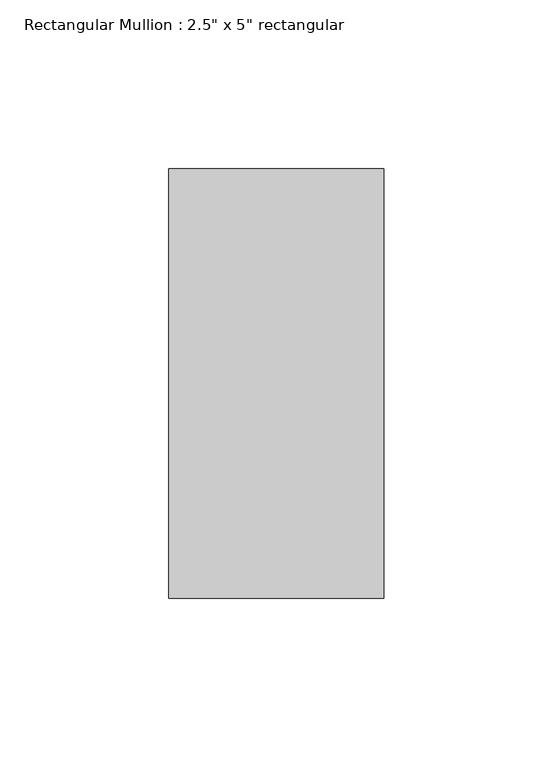
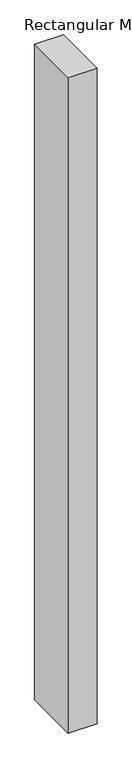
"""IFC4 building model written with IfcOpenShell, lengths in millimetres: member geometry."""

from ifc_helpers import new_model, si_unit, frame, origin, place, context, project, spatial, polyline, outline, extrude, source, transform, mapped, element, save


def member_285512ba(model_context):
    return source(origin(), model_context, "Body", "SweptSolid", [
        extrude(outline(polyline([(31.75, 63.5), (31.75, -63.5), (-31.75, -63.5), (-31.75, 63.5), (31.75, 63.5)])), frame((0.0, 0.0, -1522.1131867), z_axis=(0.0, 0.0, 1.0), x_axis=(1.0, 0.0, 0.0)), (0.0, 0.0, 1.0), 1522.1131867),
    ])


if __name__ == "__main__":
    model = new_model("IFC4")
    model_context = context("Model", 3, world=origin())
    ifc_project = project(units=[si_unit("LENGTHUNIT", "METRE", prefix="MILLI")], contexts=[model_context])
    site = spatial("IfcSite", under=ifc_project)
    building = spatial("IfcBuilding", under=site)
    placement = place(None, origin())
    member_shape = member_285512ba(model_context)
    element("IfcMember", 1, ObjectType="Rectangular Mullion : 2.5\" x 5\" rectangular", at=placement, inside=building, context=model_context, shape_type="MappedRepresentation", body=[
        mapped(member_shape, transform((0.0, 0.0, 0.0), x_axis=(1.0, 0.0, 0.0), y_axis=(0.0, 1.0, 0.0), z_axis=(0.0, 0.0, 1.0))),
    ])
    save(model, "model.ifc")

# Revit data of these elements
# Type "Rectangular Mullion : 2.5\" x 5\" rectangular"
#   built-in parameter 1007304 = 0.416667 (stored number, unit not read)
#   built-in parameter 1007301 = 0.104167 (stored number, unit not read)
#   built-in parameter 1007300 = 0.104167 (stored number, unit not read)
# Element 1 (IfcMember, "Rectangular Mullion : 2.5\" x 5\" rectangular")
#   Materials on its faces: "Aluminum"
# Materials
#   "Aluminum": class "Metal", colour RGB 247 247 247, transparency 0, Description = "Aluminum 6061", Cost = 0
